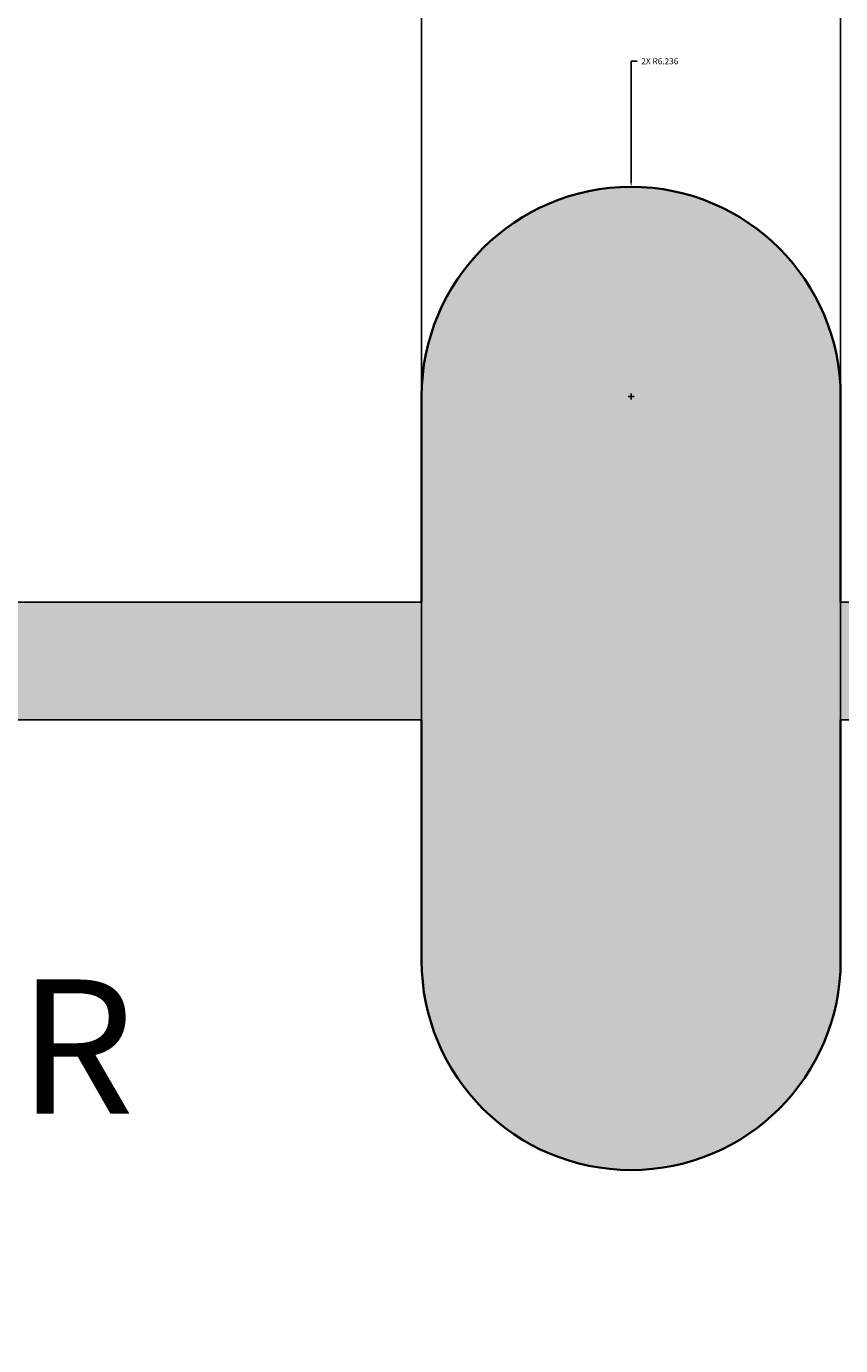
# Model space of a CAD drawing. Units: millimetres. Extents: x -11 to 280, y -4 to 208.
# Tile 10 of 55: x 67 to 91, y 87 to 126. Entities that reach past the tile are written whole.
import ezdxf
from ezdxf import colors
from ezdxf.entities.mleader import LeaderData, LeaderLine
from ezdxf.math import Vec2, Vec3

# ---------------------------------------------------------------- set-up
doc = ezdxf.new("R2010")
doc.units = ezdxf.units.MM
for name, color, linetype, lineweight in [('M-ANNO-TEXT', 7, 'Continuous', 18), ('M-DIMS', 2, 'Continuous', 18), ('M-HYDR-EQPM', 7, 'Continuous', 35), ('M-HYDR-SUCT', 7, 'Continuous', 25)]:
    doc.layers.add(name, color=color, linetype=linetype, lineweight=lineweight)
doc.layers.add('M-HYDR-SUCT-PATT', color=221, linetype='Continuous', lineweight=13, true_color=0xff7fdf)
doc.styles.get("Standard").update_dxf_attribs({"font": 'arial.ttf'})
doc.dimstyles.get("Standard").update_dxf_attribs({"dimtxt": 0.18, "dimasz": 0.18, "dimexe": 0.18, "dimexo": 0.0625, "dimgap": 0.09, "dimtad": 0, "dimtih": 1, "dimtoh": 1, "dimdec": 4, "dimzin": 0, "dimdsep": 46, "dimtxsty": 'Standard', "dimcen": 0.09, "dimadec": 0, "dimazin": 0, "dimtfac": 1, "dimtdec": 4, "dimtofl": 0, "dimtmove": 0, "dimatfit": 3, "dimfxl": 1, "dimtolj": 1, "dimtzin": 0, "dimarcsym": 0})

# ---------------------------------------------------------------- blocks, each defined once
blk = doc.blocks.new('*D5')
at = {"layer": 'Defpoints', "color": 0, "transparency": 16777216}
for p in [(24.759, 192.645), (-10.087, 11.435), (261.686, 11.435)]:
    blk.add_point(p, dxfattribs=at)
at = {"layer": 'M-DIMS', "color": 0, "lineweight": -2, "transparency": 16777216}
for p, q in [((24.696, 192.645), (-10.267, 192.645)), ((-10.087, 192.465), (-10.087, 102.222)), ((-10.087, 11.615), (-10.087, 101.858)), ((261.624, 11.435), (-10.267, 11.435))]:
    blk.add_line(p, q, dxfattribs=at)
at = {"layer": 'M-DIMS', "color": 0, "transparency": 16777216}
for points in [[(-10.117, 192.465), (-10.057, 192.465), (-10.087, 192.645)], [(-10.117, 11.615), (-10.057, 11.615), (-10.087, 11.435)]]:
    blk.add_solid(points, dxfattribs=at)
at = {"layer": 'M-DIMS', "color": 0, "transparency": 16777216, "insert": (-10.087, 102.04), "char_height": 0.18, "attachment_point": 5}
blk.add_mtext('\\A1;181.2', dxfattribs=at)
blk = doc.blocks.new('*D9')
at = {"layer": 'Defpoints', "color": 0, "transparency": 16777216}
for p in [(78.827, 207.495), (31.006, 98.021), (78.827, 98.149)]:
    blk.add_point(p, dxfattribs=at)
at = {"layer": 'M-DIMS', "color": 0, "lineweight": -2, "transparency": 16777216}
for p, q in [((31.006, 98.084), (31.006, 207.675)), ((31.186, 207.495), (54.52, 207.495)), ((78.647, 207.495), (55.313, 207.495)), ((78.827, 98.212), (78.827, 207.675))]:
    blk.add_line(p, q, dxfattribs=at)
at = {"layer": 'M-DIMS', "color": 0, "transparency": 16777216}
for points in [[(31.186, 207.525), (31.186, 207.465), (31.006, 207.495)], [(78.647, 207.525), (78.647, 207.465), (78.827, 207.495)]]:
    blk.add_solid(points, dxfattribs=at)
at = {"layer": 'M-DIMS', "color": 0, "transparency": 16777216, "insert": (54.917, 207.495), "char_height": 0.18, "attachment_point": 5}
blk.add_mtext('\\A1;47.82', dxfattribs=at)
blk = doc.blocks.new('*D11')
at = {"layer": 'Defpoints', "color": 0, "transparency": 16777216}
for p in [(118.514, 207.495), (91.3, 98.149), (118.514, 96.485)]:
    blk.add_point(p, dxfattribs=at)
at = {"layer": 'M-DIMS', "color": 0, "lineweight": -2, "transparency": 16777216}
for p, q in [((91.3, 98.212), (91.3, 207.675)), ((91.48, 207.495), (104.442, 207.495)), ((118.334, 207.495), (105.372, 207.495)), ((118.514, 96.547), (118.514, 207.675))]:
    blk.add_line(p, q, dxfattribs=at)
at = {"layer": 'M-DIMS', "color": 0, "transparency": 16777216}
for points in [[(91.48, 207.525), (91.48, 207.465), (91.3, 207.495)], [(118.334, 207.525), (118.334, 207.465), (118.514, 207.495)]]:
    blk.add_solid(points, dxfattribs=at)
at = {"layer": 'M-DIMS', "color": 0, "transparency": 16777216, "insert": (104.907, 207.495), "char_height": 0.18, "attachment_point": 5}
blk.add_mtext('\\A1;27.214', dxfattribs=at)
blk = doc.blocks.new('*D30')
at = {"layer": 'Defpoints', "color": 0, "transparency": 16777216}
for p in [(85.064, 121.182), (85.064, 114.945)]:
    blk.add_point(p, dxfattribs=at)
at = {"layer": 'M-DIMS', "color": 0, "lineweight": -2, "transparency": 16777216}
for p, q in [((85.244, 124.923), (85.064, 124.923)), ((85.064, 124.923), (85.064, 121.362)), ((84.974, 114.945), (85.154, 114.945)), ((85.064, 114.855), (85.064, 115.035))]:
    blk.add_line(p, q, dxfattribs=at)
at = {"layer": 'M-DIMS', "color": 0, "transparency": 16777216}
blk.add_solid([(85.034, 121.362), (85.094, 121.362), (85.064, 121.182)], dxfattribs=at)
at = {"layer": 'M-DIMS', "color": 0, "transparency": 16777216, "insert": (85.919, 124.923), "char_height": 0.18, "attachment_point": 5}
blk.add_mtext('\\A1;2X R6.236', dxfattribs=at)

msp = doc.modelspace()

# ---------------------------------------------------------------- hatches: boundary and pattern name
at = {"layer": 'M-HYDR-SUCT-PATT'}
h = msp.add_hatch(color=256, dxfattribs=at)
h.set_gradient(color1=(255, 127, 223), color2=(255, 127, 223), tint=1, name='INVCYLINDER')
h.paths.add_polyline_path([(91.3629, 155.4768), (91.3629, 132.4768), (58.3629, 132.4768), (58.3629, 153.9768), (54.8629, 153.9768), (54.8629, 128.9768), (94.8629, 128.9768), (94.8629, 151.9768), (205.5315, 151.9768), (205.5315, 155.4768)])
h.paths.add_polyline_path([(91.3, 114.9452, 1), (78.8273, 114.9452), (78.8273, 108.8141), (42.6453, 108.8141), (42.6453, 153.9768), (39.1453, 153.9768), (39.1453, 105.3141), (78.8273, 105.3141), (78.8273, 98.1491, 1), (91.3, 98.1491), (91.3, 105.3141), (95.5776, 105.3141), (95.5776, 108.8141), (91.3, 108.8141)])
h.paths.add_polyline_path([(228.7, 138.4081), (232.2, 138.4081), (232.2, 144.6609), (228.7, 144.6609)])
h.paths.add_polyline_path([(253.1005, 151.9768, 1), (253.1005, 155.4768), (252.6001, 155.4768), (253.5249, 153.991, -0.1401047), (253.6005, 153.7268, -0.7542249), (252.676, 153.4626), (251.4221, 155.4768), (236.9353, 155.4768), (236.9353, 151.9768)])
h.paths.add_polyline_path([(30.8182, 40.7626), (30.8182, 36.7626), (60.8182, 36.7626), (60.8182, 40.7626)])

# ---------------------------------------------------------------- linework, layer by layer
at = {"layer": 'M-HYDR-EQPM'}
for points in [[(78.8273, 108.8141), (78.8273, 114.9452)], [(91.3, 114.9452), (91.3, 108.8141)], [(78.8273, 98.1491), (78.8273, 105.3141)], [(91.3, 105.3141), (91.3, 98.1491)]]:
    msp.add_lwpolyline(points, dxfattribs=at)
for centre, start, end in [((85.0636, 114.9452), 0, 180), ((85.0636, 98.1491), 180, 0)]:
    msp.add_arc(centre, 6.2364, start, end, dxfattribs=at)
at = {"layer": 'M-HYDR-SUCT'}
for points in [[(78.8273, 105.3141), (39.1453, 105.3141), (39.1453, 153.9768)], [(78.8273, 108.8141), (42.6453, 108.8141), (42.6453, 153.9768)], [(95.5776, 108.8141), (91.3, 108.8141)], [(95.5776, 105.3141), (91.3, 105.3141)]]:
    msp.add_lwpolyline(points, dxfattribs=at)

# ---------------------------------------------------------------- dimensions: what is measured, and where the dimension line sits
at = {"layer": 'M-DIMS'}
for base, p1, p2, override, picture, middle in [((78.8273, 207.495), (31.0059, 98.0213), (78.8273, 98.1491), {"dimdec": 2, "dimlfac": 1, "dimrnd": 0, "dimzin": 0, "dimdsep": 46, "dimlunit": 2}, '*D9', (54.9166, 207.495)), ((118.5137, 207.495), (91.3, 98.1491), (118.5137, 96.4849), {"dimdec": 3, "dimlfac": 1, "dimrnd": 0, "dimzin": 0, "dimdsep": 46, "dimlunit": 2}, '*D11', (104.9068, 207.495))]:
    dim = msp.add_linear_dim(base=base, p1=p1, p2=p2, dimstyle='Standard', override=override, dxfattribs=at)
    dim.commit()
    dim.dimension.update_dxf_attribs({"geometry": picture, "text_midpoint": middle})
dim = msp.add_linear_dim(base=(-10.0865, 11.4346), p1=(24.7588, 192.645), p2=(261.6863, 11.4346), angle=90, dimstyle='Standard', override={"dimdec": 1, "dimlfac": 1, "dimrnd": 0, "dimzin": 0, "dimdsep": 46, "dimlunit": 2}, dxfattribs=at)
dim.commit()
dim.dimension.update_dxf_attribs({"geometry": '*D5', "text_midpoint": (-10.0865, 102.0398)})
dim = msp.add_radius_dim(center=(85.0636, 114.9452), mpoint=(85.064, 121.1816), text='2X <>', dimstyle='Standard', override={"dimdec": 3, "dimlfac": 1, "dimrnd": 0, "dimzin": 0, "dimdsep": 46, "dimlunit": 2}, dxfattribs=at)
dim.commit()
dim.dimension.update_dxf_attribs({"geometry": '*D30', "text_midpoint": (85.9189, 124.9234), "dimtype": 164})

# ---------------------------------------------------------------- leaders
at = {"layer": 'M-ANNO-TEXT'}
ml = msp.add_multileader_mtext('Standard', dxfattribs=at)
ml.set_content('FILTER', color=256)
ml.set_leader_properties()
ml.build(insert=Vec2(0, 0))
ctx = ml.context
ctx.base_point, ctx.plane_origin = Vec3(50.7635, 95.5863), Vec3(31.0059, 88.798)
notes = []
notes.append((ctx, [(0, (1, 1, 0), (42.7635, 95.5863), (1, 0), 8, [(0, [(31.0059, 88.798)], 0, [])])]))
ctx.mtext.insert, ctx.mtext.flow_direction = Vec3(52.7635, 97.5863), 5
for ctx, leaders in notes:
    for number, flags, end, landing, length, lines in leaders:
        leader = LeaderData()
        leader.index, (leader.has_last_leader_line, leader.has_dogleg_vector, leader.attachment_direction) = number, flags
        leader.last_leader_point, leader.dogleg_vector, leader.dogleg_length = Vec3(end), Vec3(landing), length
        for number, points, colour, breaks in lines:
            line = LeaderLine()
            line.index, line.vertices, line.color, line.breaks = number, Vec3.list(points), colors.encode_raw_color(colour), breaks
            leader.lines.append(line)
        ctx.leaders.append(leader)

doc.saveas('drawing.dxf')
